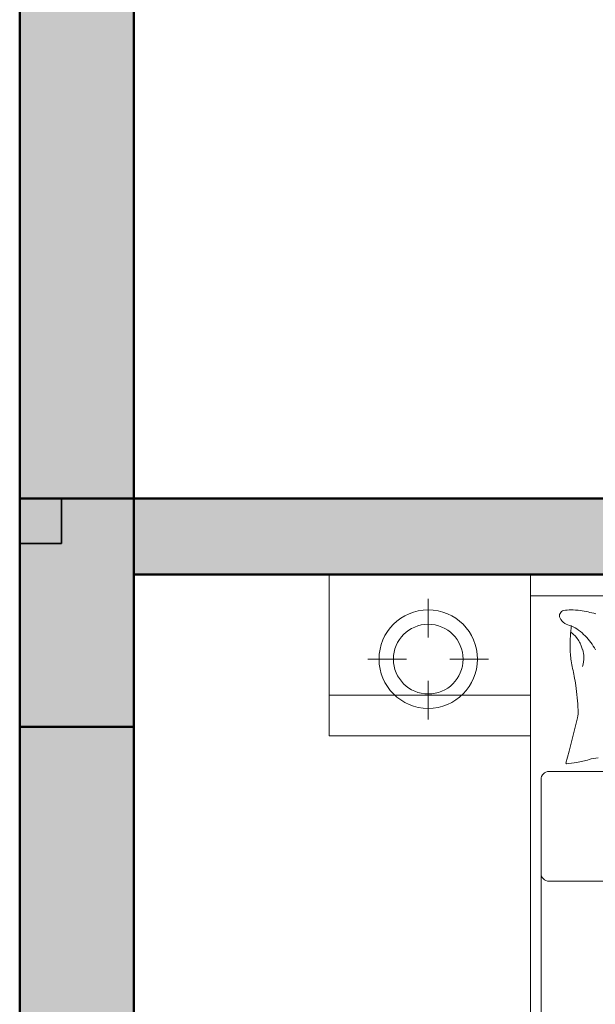
# Model space of a CAD drawing. Units: inches. Extents: x -7 to 1228, y -146 to 1091.
# Tile 9 of 88: x 60 to 105, y 453 to 531. Entities that reach past the tile are written whole.
import ezdxf

# ---------------------------------------------------------------- set-up
doc = ezdxf.new("R2010")
doc.units = ezdxf.units.IN
for name, color, linetype, lineweight in [('A-COLS', 6, 'Continuous', 35), ('A-FURN', 8, 'Continuous', 18), ('A-WALL', 7, 'Continuous', 50), ('A-WALL-PATT', 251, 'Continuous', 13)]:
    doc.layers.add(name, color=color, linetype=linetype, lineweight=lineweight)
doc.styles.add('DIM_FONT', font='SIMPLEX.shx', dxfattribs={"width": 0.8})

# ---------------------------------------------------------------- blocks, each defined once
blk = doc.blocks.new('A$C4F634EDD')
for p, q in [((0, 2.6295), (0, 2.2295)), ((0.5, 2.6295), (0, 2.6295)), ((0.5, 2.6295), (2.3, 2.6295)), ((0.5, 0.5295), (0.5, 2.6295)), ((0.5, 2.2295), (0.5, 2.6295)), ((0.2457, 2.5697), (0.2457, 2.4733)), ((0.5, 2.5771), (2.3, 2.5771)), ((0.0957, 2.4197), (0.192, 2.4197)), ((0.2994, 2.4197), (0.3957, 2.4197)), ((0.2457, 2.366), (0.2457, 2.2697)), ((0, 2.3301), (0.5, 2.3301)), ((0.5953, 2.1912), (0.616, 2.2738)), ((0, 2.2295), (0.5, 2.2295)), ((0.5878, 2.1612), (0.5953, 2.1912)), ((1.5035, 2.141), (0.5458, 2.141)), ((0.5258, 2.121), (0.5258, 0.5617)), ((0.5458, 1.8684), (1.5653, 1.8684))]:
    blk.add_line(p, q)
for radius in [0.1222, 0.0865]:
    blk.add_circle((0.2457, 2.4197), radius)
for centre, radius, start, end in [((0.5999, 2.4516), 0.0904, 90, 101.2724), ((0.5999, 2.3808), 0.1611, 81.5628, 90), ((0.5848, 2.5274), 0.0131, 101.2724, 206.5805), ((0.6036, 2.5368), 0.0342, 206.5805, 265.5998), ((0.5788, 2.2388), 0.3048, 74.256, 81.5628), ((1.0898, 2.4496), 0.4918, 173.7676, 180), ((0.5368, 2.3783), 0.1399, 45.0976, 62.7964), ((0.5462, 2.4142), 0.0899, 41.4429, 53.7359), ((0.5741, 2.4389), 0.0526, 25.3551, 41.4429), ((0.5368, 2.3783), 0.1399, 27.3988, 45.0976), ((0.8019, 2.4496), 0.204, 180, 189.6844), ((0.4851, 2.3967), 0.1511, 21.8149, 25.3551), ((0.4345, 2.3765), 0.2056, 18.7799, 21.8149), ((0.576, 2.4246), 0.0562, 0, 18.7799), ((0.5406, 2.4246), 0.0915, 345.3149, 0), ((1.4703, 2.5637), 0.882, 189.6844, 192.1984), ((0.2982, 2.3103), 0.3171, 8.0051, 12.1984), ((-0.0401, 2.2627), 0.6588, 2.6649, 8.0051), ((0.5503, 2.2902), 0.0677, 345.9548, 2.6649), ((0.6807, 2.0561), 0.1197, 96.4341, 107.3864), ((0.5887, 2.1609), 0.000917, 165.9551, 274.0829), ((0.5695, 2.4301), 0.2708, 274.0829, 279.4841), ((0.5763, 2.3896), 0.2297, 279.4841, 287.3864), ((0.5458, 2.121), 0.02, 90, 180), ((0.5458, 1.8884), 0.02, 180, 270)]:
    blk.add_arc(centre, radius, start, end)
at = {"style": 'DIM_FONT', "width": 0.8, "flags": 9}
for tag, p in [('YSIZE', (0.5, 2.6295)), ('XSIZE', (0.5, 2.6295)), ('XSIZE', (2.2985, 2.6295)), ('YSIZE', (2.2985, 2.6295))]:
    blk.add_attdef(tag, p, '', height=0.0005, dxfattribs=at)

msp = doc.modelspace()

# ---------------------------------------------------------------- hatches: boundary and pattern name
at = {"layer": 'A-COLS'}
h = msp.add_hatch(color=256, dxfattribs=at)
h.dxf.hatch_style = 1
h.paths.add_polyline_path([(60, 475), (69, 475), (69, 493), (63.289, 493), (63.289, 489.454), (60, 489.454)])
h = msp.add_hatch(color=256, dxfattribs=at)
h.dxf.hatch_style = 1
h.paths.add_polyline_path([(63.289, 489.454), (63.289, 493), (60, 493), (60, 489.454)])
at = {"layer": 'A-WALL-PATT'}
h = msp.add_hatch(color=256, dxfattribs=at)
h.dxf.hatch_style = 1
h.paths.add_polyline_path([(69, 568), (60, 568), (60, 493), (63.289, 493), (69, 493)])
h.paths.add_polyline_path([(69, 662.405), (60, 662.405), (60, 586), (69, 586)], flags=17)
h.paths.add_polyline_path([(69, 723), (184, 723), (184, 734), (179, 734), (179, 728), (69, 728), (69, 741.623), (60, 741.623), (60, 698.405), (69, 698.405)], flags=17)
h.paths.add_polyline_path([(69, 782), (231, 782), (231, 728), (231, 723), (231, 586), (236, 586), (236, 787), (69, 787), (69, 800.126), (60, 800.126), (60, 765.623), (69, 765.623)])
h.paths.add_polyline_path([(184, 842), (189, 842), (189, 848), (173, 848), (173, 842), (179, 842), (179, 787), (184, 787)])
h.paths.add_polyline_path([(118.22, 69), (69, 69), (69, 60), (118.22, 60)])
h.paths.add_polyline_path([(227, 69), (154.22, 69), (154.22, 60), (227, 60)])
h.paths.add_polyline_path([(236, 60), (232.711, 60), (227, 60), (227, 36), (236, 36)])
h.paths.add_polyline_path([(389, 60), (380, 60), (380, 36), (389, 36)])
h.paths.add_polyline_path([(384, 181), (380, 181), (380, 115), (380, 78), (384, 78)])
h.paths.add_polyline_path([(380, 115), (334.547, 115), (334.547, 109), (380, 109)])
h.paths.add_polyline_path([(274.547, 115), (236, 115), (236, 201), (232.711, 201), (231, 201), (231, 78), (236, 78), (236, 109), (274.547, 109)])
h.paths.add_polyline_path([(69, 123), (60, 123), (60, 78), (69, 78)])
h.paths.add_polyline_path([(69, 201), (60, 201), (60, 159), (69, 159)])
h.paths.add_polyline_path([(143, 219), (69, 219), (69, 213), (143, 213)], flags=17)
h.paths.add_polyline_path([(189, 219), (184, 219), (184, 274), (231, 274), (231, 219), (236, 219), (236, 279), (184, 279), (184, 297), (179, 297), (179, 279), (69, 279), (69, 290.912), (60, 290.912), (60, 262.179), (69, 262.179), (69, 274), (179, 274), (179, 219), (173, 219), (173, 213), (189, 213)])
h.paths.add_polyline_path([(69, 238.179), (60, 238.179), (60, 219), (69, 219)], flags=17)
h.paths.add_polyline_path([(69, 333), (60, 333), (60, 314.912), (69, 314.912), (69, 316.965)])
h.paths.add_polyline_path([(190, 338), (184, 338), (69, 338), (69, 333), (179, 333), (179, 327), (184, 327), (184, 333.021), (190, 333.046)])
h.paths.add_polyline_path([(69, 386.806), (60, 386.806), (60, 351), (69, 351)])
h.paths.add_polyline_path([(69, 475), (60, 475), (60, 422.806), (69, 422.806)])
h.paths.add_polyline_path([(236, 475), (231, 475), (231, 351.238), (236, 351.238)])
h.paths.add_polyline_path([(384, 475), (380, 475), (380, 362), (384, 362)])
h.paths.add_polyline_path([(547, 307), (439, 307), (439, 356), (445, 356), (445, 362), (433, 362), (433, 307), (380, 307), (380, 244), (380, 241), (384, 241), (384, 301), (433, 301), (433, 277), (439, 277), (439, 301), (547, 301)])
h.paths.add_polyline_path([(547, 241), (439, 241), (439, 247), (433, 247), (433, 235), (547, 235)])
h.paths.add_polyline_path([(450, 69), (440.286, 69), (424.889, 69), (389, 69), (389, 60), (450, 60)])
h.paths.add_polyline_path([(547, 69), (486, 69), (486, 60), (547, 60)])
h.paths.add_polyline_path([(556, 148.268), (547, 148.268), (547, 78), (556, 78)])
h.paths.add_polyline_path([(556, 223), (547, 223), (547, 195), (547, 184.268), (556, 184.268)])
h.paths.add_polyline_path([(556, 311.192), (547, 311.192), (547, 273.075), (556, 273.075)])
h.paths.add_polyline_path([(556, 344), (552.711, 344), (547, 344), (547, 335.192), (556, 335.192)])
h.paths.add_polyline_path([(556, 249.075), (547, 249.075), (547, 241), (556, 241)])
h.paths.add_polyline_path([(547, 362), (475, 362), (475, 356), (547, 356)], flags=0)
h.paths.add_polyline_path([(556, 399.621), (547, 399.621), (547, 362), (556, 362)])
h.paths.add_polyline_path([(556, 475), (547, 475), (547, 435.621), (556, 435.621)])
h.paths.add_polyline_path([(547, 493), (389, 493), (389, 487), (547, 487)])
h.paths.add_polyline_path([(380, 493), (278, 493), (278, 487), (380, 487)])
h.paths.add_polyline_path([(227, 493), (69, 493), (69, 487), (227, 487)])
h.paths.add_polyline_path([(643, 122.445), (634, 122.445), (634, 78), (643, 78)])
h.paths.add_polyline_path([(702.5, 69), (692.786, 69), (677.389, 69), (643, 69), (643, 60), (702.5, 60)])
h.paths.add_polyline_path([(798, 69), (738.5, 69), (738.5, 60), (798, 60)])
h.paths.add_polyline_path([(807, 60), (803.711, 60), (798, 60), (798, 36), (807, 36)])
h.paths.add_polyline_path([(807, 109), (846.751, 109), (846.751, 115), (807, 115), (807, 159), (802, 159), (802, 78), (807, 78)])
h.paths.add_polyline_path([(807, 201), (802, 201), (802, 195), (807, 195)])
h.paths.add_polyline_path([(643, 201), (634, 201), (634, 158.445), (643, 158.445)])
h.paths.add_polyline_path([(756, 225), (751, 225), (751, 219), (643, 219), (643, 213), (756, 213)])
h.paths.add_polyline_path([(643, 240.848), (634, 240.848), (634, 219), (643, 219)])
h.paths.add_polyline_path([(643, 274), (643, 288.629), (634, 288.629), (634, 264.848), (643, 264.848)])
h.paths.add_polyline_path([(802, 279), (756, 279), (756, 297), (751, 297), (751, 279), (643, 279), (643, 274), (751, 274), (751, 255), (756, 255), (756, 274), (802, 274)])
h.paths.add_polyline_path([(807, 333), (803.711, 333), (802, 333), (802, 279), (802, 274), (802, 219), (807, 219)])
h.paths.add_polyline_path([(956, 182), (951, 182), (951, 115), (906.751, 115), (906.751, 109), (951, 109), (951, 78), (956, 78)])
h.paths.add_polyline_path([(960, 60), (951, 60), (951, 36), (960, 36)])
h.paths.add_polyline_path([(1021, 69), (1005.781, 69), (960, 69), (960, 60), (1021, 60)])
h.paths.add_polyline_path([(956, 224), (951, 224), (951, 218), (956, 218)])
h.paths.add_polyline_path([(956, 302), (1004, 302), (1004, 278), (1010, 278), (1010, 302), (1118, 302), (1118, 290.809), (1127, 290.809), (1127, 326.968), (1118, 326.968), (1118, 320.966), (1118, 307), (1010, 307), (1010, 356), (1016, 356), (1016, 362), (1004, 362), (1004, 307), (951, 307), (951, 244), (951, 242), (954.289, 242), (956, 242)])
h.paths.add_polyline_path([(643, 333), (634, 333), (634, 312.629), (643, 312.629), (643, 316.965)])
h.paths.add_polyline_path([(756, 338), (643, 338), (643, 333), (751, 333), (751, 327), (756, 327)])
h.paths.add_polyline_path([(643, 388), (634, 388), (634, 351), (643, 351)])
h.paths.add_polyline_path([(807, 357), (802, 357), (802, 351), (807, 351)])
h.paths.add_polyline_path([(807, 475), (802, 475), (802, 393), (807, 393)])
h.paths.add_polyline_path([(643, 475), (634, 475), (634, 424), (643, 424)])
h.paths.add_polyline_path([(798, 493), (643, 493), (643, 487), (798, 487)])
h.paths.add_polyline_path([(634, 493), (556, 493), (556, 487), (634, 487)])
h.paths.add_polyline_path([(813, 493), (807, 493), (807, 487), (813, 487)])
h.paths.add_polyline_path([(951, 493), (849, 493), (849, 487), (951, 487)])
h.paths.add_polyline_path([(956, 484), (951, 484), (951, 374), (956, 374)])
h.paths.add_polyline_path([(1109, 493), (969, 493), (969, 487), (1109, 487)])
h.paths.add_polyline_path([(1127, 484), (1118, 484), (1118, 450.641), (1127, 450.641)])
h.paths.add_polyline_path([(1127, 414.641), (1118, 414.641), (1118, 365), (1127, 365)])
h.paths.add_polyline_path([(1109, 362), (1046, 362), (1046, 356), (1109, 356)], flags=17)
h.paths.add_polyline_path([(1127, 356), (1123.454, 356), (1118, 356), (1118, 350.968), (1127, 350.968)], flags=0)
h.paths.add_polyline_path([(1127, 266.809), (1118, 266.809), (1118, 262.361), (1118, 242), (1127, 242)], flags=17)
h.paths.add_polyline_path([(1118, 242), (1010, 242), (1010, 248), (1004, 248), (1004, 237), (1118, 237)])
h.paths.add_polyline_path([(1127, 224), (1118, 224), (1118, 170), (1127, 170)])
h.paths.add_polyline_path([(1127, 134), (1118, 134), (1118, 78), (1127, 78)])
h.paths.add_polyline_path([(1118, 69), (1057, 69), (1057, 60), (1118, 60)])
h.paths.add_polyline_path([(227, 571.546), (227, 574), (69, 574), (69, 568), (227, 568)])
h.paths.add_polyline_path([(380, 571.546), (380, 574), (278, 574), (278, 568), (380, 568)])
h.paths.add_polyline_path([(242, 574), (236, 574), (236, 568), (242, 568)])
h.paths.add_polyline_path([(547, 571.546), (547, 574), (389, 574), (389, 568), (547, 568)])
h.paths.add_polyline_path([(384, 733), (380, 733), (380, 586), (384, 586)])
h.paths.add_polyline_path([(556, 646), (634, 646), (634, 655), (547, 655), (547, 586), (556, 586)])
h.paths.add_polyline_path([(634, 574), (556, 574), (556, 568), (634, 568)])
h.paths.add_polyline_path([(643, 655), (634, 655), (634, 586), (643, 586)])
h.paths.add_polyline_path([(798, 574), (643, 574), (643, 568), (798, 568)])
h.paths.add_polyline_path([(643, 663.854), (634, 663.854), (634, 655), (643, 655)])
h.paths.add_polyline_path([(556, 676.967), (547, 676.967), (547, 655), (556, 655)])
h.paths.add_polyline_path([(556, 733), (547, 733), (547, 712.967), (556, 712.967)])
h.paths.add_polyline_path([(643, 710), (634, 710), (634, 699.854), (643, 699.854)])
h.paths.add_polyline_path([(807, 668), (802, 668), (802, 586), (807, 586)])
h.paths.add_polyline_path([(951, 574), (849, 574), (849, 568), (951, 568)])
h.paths.add_polyline_path([(956, 691), (951, 691), (951, 577), (956, 577)])
h.paths.add_polyline_path([(1109, 574), (969, 574), (969, 568), (1109, 568)])
h.paths.add_polyline_path([(1127, 643.403), (1118, 643.403), (1118, 577), (1127, 577)])
h.paths.add_polyline_path([(1127, 568), (1123.454, 568), (1118, 568), (1118, 493), (1127, 493)])
h.paths.add_polyline_path([(1127, 733), (1118, 733), (1118, 679.403), (1127, 679.403)])
h.paths.add_polyline_path([(1127, 777.348), (1118, 777.348), (1118, 770.035), (1118, 751), (1127, 751)], flags=17)
h.paths.add_polyline_path([(1118, 751), (1010, 751), (1010, 757), (1004, 757), (1004, 745), (1118, 745)])
h.paths.add_polyline_path([(956, 811), (1004, 811), (1004, 787), (1010, 787), (1010, 811), (1017.874, 811), (1017.874, 811.627, -0.414214), (1018.247, 812), (1031.978, 812, -0.414214), (1032.351, 811.627), (1032.351, 811), (1118, 811), (1118, 801.348), (1127, 801.348), (1127, 834.685), (1118, 834.685), (1118, 830.238), (1118, 817), (1010, 817), (1010, 866), (1016, 866), (1016, 872), (1004, 872), (1004, 817), (956, 817), (956, 866), (951, 866), (951, 751), (954.289, 751), (956, 751)])
h.paths.add_polyline_path([(1118, 872), (1046, 872), (1046, 866), (1118, 866)], flags=17)
h.paths.add_polyline_path([(1127, 924.711), (1118, 924.711), (1118, 884), (1127, 884)])
h.paths.add_polyline_path([(1127, 866), (1123.711, 866), (1118, 866), (1118, 858.685), (1127, 858.685)], flags=17)
h.paths.add_polyline_path([(956, 983), (951, 983), (951, 952), (807, 952), (807, 983), (802, 983), (802, 902), (807, 902), (807, 946), (951, 946), (951, 884), (956, 884)])
h.paths.add_polyline_path([(807, 842), (802, 842), (802, 787), (756, 787), (756, 806), (751, 806), (751, 787), (643, 787), (643, 782), (751, 782), (751, 764), (756, 764), (756, 782), (802, 782), (802, 728), (807, 728)])
h.paths.add_polyline_path([(756, 848), (643, 848), (643, 842), (751, 842), (751, 836), (756, 836)])
h.paths.add_polyline_path([(756, 734), (751, 734), (751, 728), (643, 728), (643, 723), (756, 723)])
h.paths.add_polyline_path([(643, 749.791), (634, 749.791), (634, 728), (637.289, 728), (643, 728)])
h.paths.add_polyline_path([(643, 805.405), (634, 805.405), (634, 773.791), (643, 773.791)])
h.paths.add_polyline_path([(643, 896.663), (634, 896.663), (634, 860), (637.289, 860), (643, 860)])
h.paths.add_polyline_path([(643, 842), (634, 842), (634, 829.405), (643, 829.405)])
h.paths.add_polyline_path([(643, 983), (634, 983), (634, 932.663), (643, 932.663)])
h.paths.add_polyline_path([(1127, 983), (1118, 983), (1118, 960.711), (1127, 960.711)])
h.paths.add_polyline_path([(1118, 1001), (1077.525, 1001), (1077.525, 992), (1118, 992)])
h.paths.add_polyline_path([(1041.525, 1001), (960, 1001), (960, 992), (1041.525, 992)])
h.paths.add_polyline_path([(960, 1025), (951, 1025), (951, 1001), (954.289, 1001), (960, 1001)])
h.paths.add_polyline_path([(807, 1025), (798, 1025), (798, 1001), (807, 1001)])
h.paths.add_polyline_path([(798, 1001), (738.5, 1001), (738.5, 992), (798, 992)])
h.paths.add_polyline_path([(702.5, 1001), (643, 1001), (643, 992), (702.5, 992)])
h.paths.add_polyline_path([(547, 1001), (499.113, 1001), (499.113, 992), (547, 992)])
h.paths.add_polyline_path([(463.113, 1001), (389, 1001), (389, 992), (463.113, 992)])
h.paths.add_polyline_path([(389, 1025), (380, 1025), (380, 1022), (380, 1001), (383.289, 1001), (389, 1001)])
h.paths.add_polyline_path([(236, 1025), (227, 1025), (227, 1001), (236, 1001)])
h.paths.add_polyline_path([(236, 983), (231, 983), (231, 860), (236, 860)])
h.paths.add_polyline_path([(274.547, 952), (236, 952), (236, 946), (274.547, 946)])
h.paths.add_polyline_path([(380, 952), (334.547, 952), (334.547, 946), (380, 946)])
h.paths.add_polyline_path([(384, 983), (380, 983), (380, 884), (383.289, 884), (384, 884)])
h.paths.add_polyline_path([(227, 1001), (155.012, 1001), (155.012, 992), (162.875, 992), (227, 992)])
h.paths.add_polyline_path([(119.012, 1001), (69, 1001), (69, 992), (119.012, 992)])
h.paths.add_polyline_path([(69, 983), (60, 983), (60, 922.987), (69, 922.987)])
h.paths.add_polyline_path([(69, 886.987), (60, 886.987), (60, 860), (63.289, 860), (69, 860)])
h.paths.add_polyline_path([(143, 848), (69, 848), (69, 842), (143, 842)])

# ---------------------------------------------------------------- linework, layer by layer
at = {"layer": 'A-COLS'}
msp.add_lwpolyline([(60, 493), (63.289, 493), (63.289, 489.454), (60, 489.454)], close=True, dxfattribs=at)
at = {"layer": 'A-WALL'}
for p, q in [((60, 1001), (60, 60)), ((69, 568), (69, 279)), ((231, 493), (60, 493)), ((60, 493), (69, 493)), ((60, 475), (60, 493)), ((69, 493), (69, 475)), ((231, 487), (69, 487)), ((69, 338), (69, 487)), ((69, 475), (60, 475))]:
    msp.add_line(p, q, dxfattribs=at)

# ---------------------------------------------------------------- block references
at = {"layer": 'A-FURN', "xscale": 31.78426361944092, "yscale": 31.78426361944092, "zscale": 31.78426361944092}
msp.add_blockref('A$C4F634EDD', (84.435, 403.423), dxfattribs=at)

doc.saveas('drawing.dxf')
